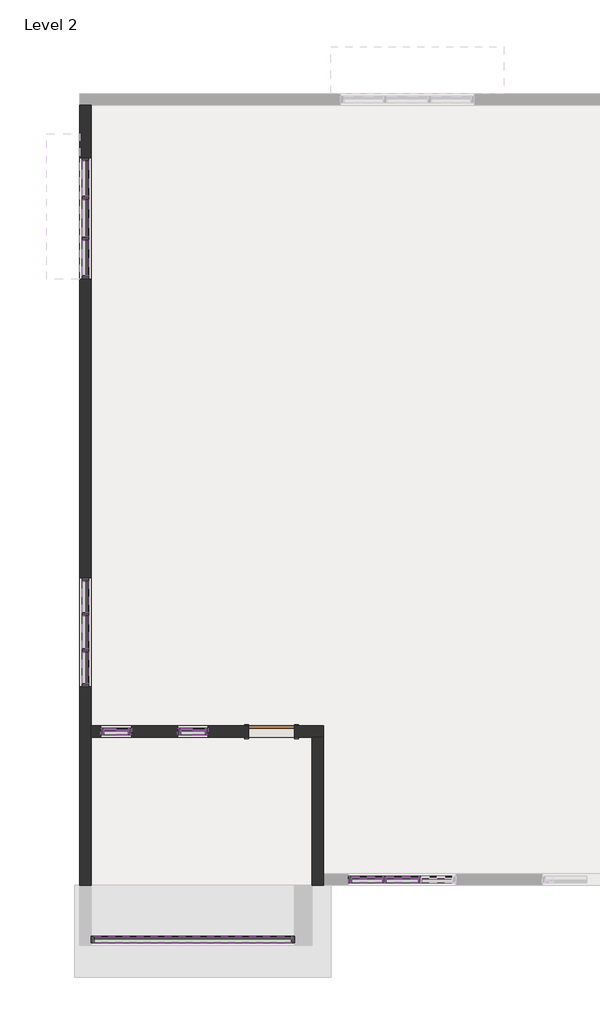
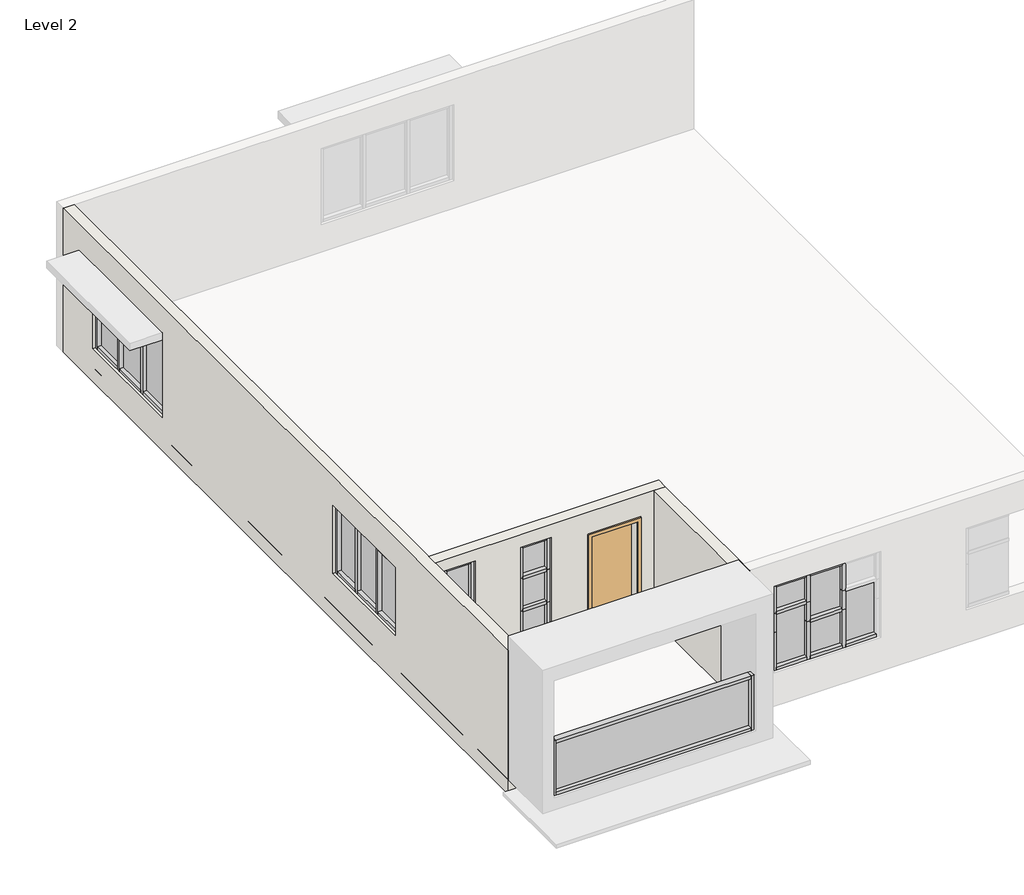
# One storey, part 1 of 2: 60 members, 18 plates, 3 walls, 1 door.
"""IFC4 building model written with IfcOpenShell, lengths in millimetres."""

from ifc_helpers import new_model, si_unit, frame, origin, place, context, project, spatial, polyline, outline, extrude, faceted_brep, transform, mapped, element, save
from components import door_a90ba1ad, member_3f0e0172, member_5215b92c, member_e53b78c9, member_f8dc38bf, member_504574e5, member_b70ee1cc, member_323df77c, member_86d06fe4, member_c0b2eca9, member_1f059faf, member_ce3cb600, member_25d88653, member_13f6f031, member_d2428cc8, member_166502d3, member_d74631f0, member_63be31b3, member_891d357d, member_df93ad89, member_28ac88d2, member_2030dc42, member_297e028d, member_b5a88f55, member_6ca94d07, member_46c3daae, system_panel_glazed_bdd26bb3, system_panel_glazed_84c2177b, system_panel_glazed_04707b35, system_panel_glazed_fe1d3f05, system_panel_glazed_483907af, system_panel_glazed_5a74f323, system_panel_glazed_03a03fc4, system_panel_glazed_c2563f89, system_panel_glazed_d3cf7d22, system_panel_glazed_f04aca20, system_panel_glazed_b3daaad5, system_panel_glazed_3e14b5a9, system_panel_glazed_68555a4f, system_panel_glazed_82e5a723

model = new_model("IFC4")

# Units and contexts
model_context = context("Model", 3, world=origin())
ifc_project = project(units=[si_unit("LENGTHUNIT", "METRE", prefix="MILLI")], contexts=[model_context])

# Site, building, storey
site = spatial("IfcSite", under=ifc_project)
building = spatial("IfcBuilding", under=site)
storey = spatial("IfcBuildingStorey", under=building, Name="Level 2", Elevation=3048.0)

# Door
placement = place(None, origin())
door_shape = door_a90ba1ad(model_context)
element("IfcDoor", 1, ObjectType="Single-Flush : 36\" x 84\"", at=placement, inside=storey, context=model_context, shape_type="MappedRepresentation", body=[
    mapped(door_shape, transform((-18035.6161422, -11856.2171312, 3429.0), x_axis=(-1.0, 0.0, 0.0), y_axis=(0.0, -1.0, 0.0), z_axis=(0.0, 0.0, 1.0))),
])

# Members
element("IfcMember", 2, ObjectType="Rectangular Mullion : 2.5\" x 5\" rectangular", at=placement, inside=storey, context=model_context, shape_type="SweptSolid", body=[
    extrude(outline(polyline([(-21553.5161422, -16047.2171312), (-21553.5161422, -15920.2171312), (-17641.9161422, -15920.2171312), (-17641.9161422, -16047.2171312), (-21553.5161422, -16047.2171312)])), frame((0.0, 0.0, 3616.9897637), z_axis=(0.0, 0.0, 1.0), x_axis=(1.0, 0.0, 0.0)), (0.0, 0.0, 1.0), 63.5),
])
member_shape = member_3f0e0172(model_context)
element("IfcMember", 3, ObjectType="Rectangular Mullion : 2.5\" x 5\" rectangular", at=placement, inside=storey, context=model_context, shape_type="MappedRepresentation", body=[
    mapped(member_shape, transform((-15057.4661422, -14789.9171312, 3757.8785057), x_axis=(0.0, 0.0, -1.0), y_axis=(0.0, -1.0, 0.0), z_axis=(-1.0, 0.0, 0.0))),
])
element("IfcMember", 4, ObjectType="Rectangular Mullion : 2.5\" x 5\" rectangular", at=placement, inside=storey, context=model_context, shape_type="MappedRepresentation", body=[
    mapped(member_shape, transform((-16448.1161422, -14789.9171312, 3757.8785057), x_axis=(0.0, 0.0, -1.0), y_axis=(0.0, -1.0, 0.0), z_axis=(-1.0, 0.0, 0.0))),
])
element("IfcMember", 5, ObjectType="Rectangular Mullion : 2.5\" x 5\" rectangular", at=placement, inside=storey, context=model_context, shape_type="MappedRepresentation", body=[
    mapped(member_shape, transform((-15832.1661422, -14789.9171312, 5583.6799972), x_axis=(0.0, 0.0, 1.0), y_axis=(0.0, -1.0, 0.0), z_axis=(1.0, 0.0, 0.0))),
])
member_2_shape = member_5215b92c(model_context)
element("IfcMember", 6, ObjectType="Rectangular Mullion : 2.5\" x 5\" rectangular", at=placement, inside=storey, context=model_context, shape_type="MappedRepresentation", body=[
    mapped(member_2_shape, transform((-15768.6661422, -14789.9171312, 3757.8785057), x_axis=(0.0, 0.0, -1.0), y_axis=(0.0, -1.0, 0.0), z_axis=(-1.0, 0.0, 0.0))),
])
element("IfcMember", 7, ObjectType="Rectangular Mullion : 2.5\" x 5\" rectangular", at=placement, inside=storey, context=model_context, shape_type="MappedRepresentation", body=[
    mapped(member_2_shape, transform((-15120.9661422, -14789.9171312, 5583.6799972), x_axis=(0.0, 0.0, 1.0), y_axis=(0.0, -1.0, 0.0), z_axis=(1.0, 0.0, 0.0))),
])
member_3_shape = member_e53b78c9(model_context)
element("IfcMember", 8, ObjectType="Rectangular Mullion : 2.5\" x 5\" rectangular", at=placement, inside=storey, context=model_context, shape_type="MappedRepresentation", body=[
    mapped(member_3_shape, transform((-15120.9661422, -14789.9171312, 4569.3458353), x_axis=(0.0, 0.0, 1.0), y_axis=(0.0, -1.0, 0.0), z_axis=(1.0, 0.0, 0.0))),
])
member_4_shape = member_f8dc38bf(model_context)
element("IfcMember", 9, ObjectType="Rectangular Mullion : 2.5\" x 5\" rectangular", at=placement, inside=storey, context=model_context, shape_type="MappedRepresentation", body=[
    mapped(member_4_shape, transform((-15832.1661422, -14789.9171312, 4975.0795001), x_axis=(0.0, 0.0, 1.0), y_axis=(0.0, -1.0, 0.0), z_axis=(1.0, 0.0, 0.0))),
])
member_5_shape = member_504574e5(model_context)
element("IfcMember", 10, ObjectType="Rectangular Mullion : 2.5\" x 5\" rectangular", at=placement, inside=storey, context=model_context, shape_type="MappedRepresentation", body=[
    mapped(member_5_shape, transform((-21426.5161422, -11856.2171312, 4991.9456117), x_axis=(-1.0, 0.0, 0.0), y_axis=(0.0, -1.0, 0.0), z_axis=(0.0, 0.0, 1.0))),
])
member_6_shape = member_b70ee1cc(model_context)
element("IfcMember", 11, ObjectType="Rectangular Mullion : 2.5\" x 5\" rectangular", at=placement, inside=storey, context=model_context, shape_type="MappedRepresentation", body=[
    mapped(member_6_shape, transform((-21426.5161422, -11856.2171312, 5855.5456117), x_axis=(-1.0, 0.0, 0.0), y_axis=(0.0, -1.0, 0.0), z_axis=(0.0, 0.0, 1.0))),
])
member_7_shape = member_323df77c(model_context)
element("IfcMember", 12, ObjectType="Rectangular Mullion : 2.5\" x 5\" rectangular", at=placement, inside=storey, context=model_context, shape_type="MappedRepresentation", body=[
    mapped(member_7_shape, transform((-20880.4161422, -11856.2171312, 4991.9456117), x_axis=(0.0, 0.0, 1.0), y_axis=(0.0, -1.0, 0.0), z_axis=(1.0, 0.0, 0.0))),
])
element("IfcMember", 13, ObjectType="Rectangular Mullion : 2.5\" x 5\" rectangular", at=placement, inside=storey, context=model_context, shape_type="MappedRepresentation", body=[
    mapped(member_7_shape, transform((-20880.4161422, -11856.2171312, 4416.0583974), x_axis=(0.0, 0.0, 1.0), y_axis=(0.0, -1.0, 0.0), z_axis=(1.0, 0.0, 0.0))),
])
element("IfcMember", 14, ObjectType="Rectangular Mullion : 2.5\" x 5\" rectangular", at=placement, inside=storey, context=model_context, shape_type="MappedRepresentation", body=[
    mapped(member_7_shape, transform((-19356.4161422, -11856.2171312, 5127.093488), x_axis=(0.0, 0.0, 1.0), y_axis=(0.0, -1.0, 0.0), z_axis=(1.0, 0.0, 0.0))),
])
element("IfcMember", 15, ObjectType="Rectangular Mullion : 2.5\" x 5\" rectangular", at=placement, inside=storey, context=model_context, shape_type="MappedRepresentation", body=[
    mapped(member_7_shape, transform((-19356.4161422, -11856.2171312, 4429.6158671), x_axis=(0.0, 0.0, 1.0), y_axis=(0.0, -1.0, 0.0), z_axis=(1.0, 0.0, 0.0))),
])
member_8_shape = member_86d06fe4(model_context)
element("IfcMember", 16, ObjectType="Rectangular Mullion : 2.5\" x 5\" rectangular", at=placement, inside=storey, context=model_context, shape_type="MappedRepresentation", body=[
    mapped(member_8_shape, transform((-20880.4161422, -11856.2171312, 5855.5456117), x_axis=(0.0, 0.0, 1.0), y_axis=(0.0, -1.0, 0.0), z_axis=(1.0, 0.0, 0.0))),
])
element("IfcMember", 17, ObjectType="Rectangular Mullion : 2.5\" x 5\" rectangular", at=placement, inside=storey, context=model_context, shape_type="MappedRepresentation", body=[
    mapped(member_8_shape, transform((-19356.4161422, -11856.2171312, 5824.5711089), x_axis=(0.0, 0.0, 1.0), y_axis=(0.0, -1.0, 0.0), z_axis=(1.0, 0.0, 0.0))),
])
element("IfcMember", 18, ObjectType="Rectangular Mullion : 2.5\" x 5\" rectangular", at=placement, inside=storey, context=model_context, shape_type="MappedRepresentation", body=[
    mapped(member_5_shape, transform((-20816.9161422, -11856.2171312, 4416.0583974), x_axis=(1.0, 0.0, 0.0), y_axis=(0.0, -1.0, 0.0), z_axis=(0.0, 0.0, -1.0))),
])
element("IfcMember", 19, ObjectType="Rectangular Mullion : 2.5\" x 5\" rectangular", at=placement, inside=storey, context=model_context, shape_type="MappedRepresentation", body=[
    mapped(member_6_shape, transform((-20816.9161422, -11856.2171312, 4991.9456117), x_axis=(1.0, 0.0, 0.0), y_axis=(0.0, -1.0, 0.0), z_axis=(0.0, 0.0, -1.0))),
])
element("IfcMember", 20, ObjectType="Rectangular Mullion : 2.5\" x 5\" rectangular", at=placement, inside=storey, context=model_context, shape_type="MappedRepresentation", body=[
    mapped(member_8_shape, transform((-21363.0161422, -11856.2171312, 3840.1711831), x_axis=(0.0, 0.0, -1.0), y_axis=(0.0, -1.0, 0.0), z_axis=(-1.0, 0.0, 0.0))),
])
element("IfcMember", 21, ObjectType="Rectangular Mullion : 2.5\" x 5\" rectangular", at=placement, inside=storey, context=model_context, shape_type="MappedRepresentation", body=[
    mapped(member_8_shape, transform((-19839.0161422, -11856.2171312, 3732.1382463), x_axis=(0.0, 0.0, -1.0), y_axis=(0.0, -1.0, 0.0), z_axis=(-1.0, 0.0, 0.0))),
])
element("IfcMember", 22, ObjectType="Rectangular Mullion : 2.5\" x 5\" rectangular", at=placement, inside=storey, context=model_context, shape_type="MappedRepresentation", body=[
    mapped(member_5_shape, transform((-21426.5161422, -11856.2171312, 4416.0583974), x_axis=(-1.0, 0.0, 0.0), y_axis=(0.0, -1.0, 0.0), z_axis=(0.0, 0.0, 1.0))),
])
element("IfcMember", 23, ObjectType="Rectangular Mullion : 2.5\" x 5\" rectangular", at=placement, inside=storey, context=model_context, shape_type="MappedRepresentation", body=[
    mapped(member_5_shape, transform((-20816.9161422, -11856.2171312, 3840.1711831), x_axis=(1.0, 0.0, 0.0), y_axis=(0.0, -1.0, 0.0), z_axis=(0.0, 0.0, -1.0))),
])
member_9_shape = member_c0b2eca9(model_context)
element("IfcMember", 24, ObjectType="Rectangular Mullion : 2.5\" x 5\" rectangular", at=placement, inside=storey, context=model_context, shape_type="MappedRepresentation", body=[
    mapped(member_9_shape, transform((-19902.5161422, -11856.2171312, 5824.5711089), x_axis=(-1.0, 0.0, 0.0), y_axis=(0.0, -1.0, 0.0), z_axis=(0.0, 0.0, 1.0))),
])
element("IfcMember", 25, ObjectType="Rectangular Mullion : 2.5\" x 5\" rectangular", at=placement, inside=storey, context=model_context, shape_type="MappedRepresentation", body=[
    mapped(member_9_shape, transform((-19902.5161422, -11856.2171312, 5127.093488), x_axis=(-1.0, 0.0, 0.0), y_axis=(0.0, -1.0, 0.0), z_axis=(0.0, 0.0, 1.0))),
])
element("IfcMember", 26, ObjectType="Rectangular Mullion : 2.5\" x 5\" rectangular", at=placement, inside=storey, context=model_context, shape_type="MappedRepresentation", body=[
    mapped(member_9_shape, transform((-19902.5161422, -11856.2171312, 4429.6158671), x_axis=(-1.0, 0.0, 0.0), y_axis=(0.0, -1.0, 0.0), z_axis=(0.0, 0.0, 1.0))),
])
element("IfcMember", 27, ObjectType="Rectangular Mullion : 2.5\" x 5\" rectangular", at=placement, inside=storey, context=model_context, shape_type="MappedRepresentation", body=[
    mapped(member_9_shape, transform((-19292.9161422, -11856.2171312, 4429.6158671), x_axis=(1.0, 0.0, 0.0), y_axis=(0.0, -1.0, 0.0), z_axis=(0.0, 0.0, -1.0))),
])
element("IfcMember", 28, ObjectType="Rectangular Mullion : 2.5\" x 5\" rectangular", at=placement, inside=storey, context=model_context, shape_type="MappedRepresentation", body=[
    mapped(member_9_shape, transform((-19292.9161422, -11856.2171312, 5127.093488), x_axis=(1.0, 0.0, 0.0), y_axis=(0.0, -1.0, 0.0), z_axis=(0.0, 0.0, -1.0))),
])
element("IfcMember", 29, ObjectType="Rectangular Mullion : 2.5\" x 5\" rectangular", at=placement, inside=storey, context=model_context, shape_type="MappedRepresentation", body=[
    mapped(member_9_shape, transform((-19292.9161422, -11856.2171312, 3732.1382463), x_axis=(1.0, 0.0, 0.0), y_axis=(0.0, -1.0, 0.0), z_axis=(0.0, 0.0, -1.0))),
])
member_10_shape = member_1f059faf(model_context)
element("IfcMember", 30, ObjectType="Rectangular Mullion : 2.5\" x 5\" rectangular", at=placement, inside=storey, context=model_context, shape_type="MappedRepresentation", body=[
    mapped(member_10_shape, transform((-16511.6161422, -14789.9171312, 4569.3458353), x_axis=(-1.0, 0.0, 0.0), y_axis=(0.0, -1.0, 0.0), z_axis=(0.0, 0.0, 1.0))),
])
member_11_shape = member_ce3cb600(model_context)
element("IfcMember", 31, ObjectType="Rectangular Mullion : 2.5\" x 5\" rectangular", at=placement, inside=storey, context=model_context, shape_type="MappedRepresentation", body=[
    mapped(member_11_shape, transform((-15800.4161422, -14789.9171312, 4975.0795001), x_axis=(1.0, 0.0, 0.0), y_axis=(0.0, -1.0, 0.0), z_axis=(0.0, 0.0, -1.0))),
])
element("IfcMember", 32, ObjectType="Rectangular Mullion : 2.5\" x 5\" rectangular", at=placement, inside=storey, context=model_context, shape_type="MappedRepresentation", body=[
    mapped(member_11_shape, transform((-15089.2161422, -14789.9171312, 4975.0795001), x_axis=(1.0, 0.0, 0.0), y_axis=(0.0, -1.0, 0.0), z_axis=(0.0, 0.0, -1.0))),
])
member_12_shape = member_25d88653(model_context)
element("IfcMember", 33, ObjectType="Rectangular Mullion : 2.5\" x 5\" rectangular", at=placement, inside=storey, context=model_context, shape_type="MappedRepresentation", body=[
    mapped(member_12_shape, transform((-16511.6161422, -14789.9171312, 4975.0795001), x_axis=(-1.0, 0.0, 0.0), y_axis=(0.0, -1.0, 0.0), z_axis=(0.0, 0.0, 1.0))),
])
member_13_shape = member_13f6f031(model_context)
element("IfcMember", 34, ObjectType="Rectangular Mullion : 2.5\" x 5\" rectangular", at=placement, inside=storey, context=model_context, shape_type="MappedRepresentation", body=[
    mapped(member_13_shape, transform((-16511.6161422, -14789.9171312, 5583.6799972), x_axis=(-1.0, 0.0, 0.0), y_axis=(0.0, -1.0, 0.0), z_axis=(0.0, 0.0, 1.0))),
])
member_14_shape = member_d2428cc8(model_context)
element("IfcMember", 35, ObjectType="Rectangular Mullion : 2.5\" x 5\" rectangular", at=placement, inside=storey, context=model_context, shape_type="MappedRepresentation", body=[
    mapped(member_14_shape, transform((-15800.4161422, -14789.9171312, 4569.3458353), x_axis=(1.0, 0.0, 0.0), y_axis=(0.0, -1.0, 0.0), z_axis=(0.0, 0.0, -1.0))),
])
element("IfcMember", 36, ObjectType="Rectangular Mullion : 2.5\" x 5\" rectangular", at=placement, inside=storey, context=model_context, shape_type="MappedRepresentation", body=[
    mapped(member_14_shape, transform((-15089.2161422, -14789.9171312, 4569.3458353), x_axis=(1.0, 0.0, 0.0), y_axis=(0.0, -1.0, 0.0), z_axis=(0.0, 0.0, -1.0))),
])
member_15_shape = member_166502d3(model_context)
element("IfcMember", 37, ObjectType="Rectangular Mullion : 2.5\" x 5\" rectangular", at=placement, inside=storey, context=model_context, shape_type="MappedRepresentation", body=[
    mapped(member_15_shape, transform((-15800.4161422, -14789.9171312, 3757.8785057), x_axis=(1.0, 0.0, 0.0), y_axis=(0.0, -1.0, 0.0), z_axis=(0.0, 0.0, -1.0))),
])
element("IfcMember", 38, ObjectType="Rectangular Mullion : 2.5\" x 5\" rectangular", at=placement, inside=storey, context=model_context, shape_type="MappedRepresentation", body=[
    mapped(member_15_shape, transform((-15089.2161422, -14789.9171312, 3757.8785057), x_axis=(1.0, 0.0, 0.0), y_axis=(0.0, -1.0, 0.0), z_axis=(0.0, 0.0, -1.0))),
])
member_16_shape = member_d74631f0(model_context)
element("IfcMember", 39, ObjectType="Rectangular Mullion : 2.5\" x 5\" rectangular", at=placement, inside=storey, context=model_context, shape_type="MappedRepresentation", body=[
    mapped(member_16_shape, transform((-21617.0161422, -15983.7171312, 4779.1840663), x_axis=(-1.0, 0.0, 0.0), y_axis=(0.0, -1.0, 0.0), z_axis=(0.0, 0.0, 1.0))),
])
member_17_shape = member_63be31b3(model_context)
element("IfcMember", 40, ObjectType="Rectangular Mullion : 2.5\" x 5\" rectangular", at=placement, inside=storey, context=model_context, shape_type="MappedRepresentation", body=[
    mapped(member_17_shape, transform((-17641.9161422, -15983.7171312, 4779.1840663), x_axis=(0.0, 0.0, 1.0), y_axis=(0.0, -1.0, 0.0), z_axis=(1.0, 0.0, 0.0))),
])
element("IfcMember", 41, ObjectType="Rectangular Mullion : 2.5\" x 5\" rectangular", at=placement, inside=storey, context=model_context, shape_type="MappedRepresentation", body=[
    mapped(member_16_shape, transform((-17578.4161422, -15983.7171312, 3616.9897637), x_axis=(1.0, 0.0, 0.0), y_axis=(0.0, -1.0, 0.0), z_axis=(0.0, 0.0, -1.0))),
])
member_18_shape = member_891d357d(model_context)
element("IfcMember", 42, ObjectType="Rectangular Mullion : 2.5\" x 5\" rectangular", at=placement, inside=storey, context=model_context, shape_type="MappedRepresentation", body=[
    mapped(member_18_shape, transform((-21731.3161422, -2046.5619465, 5394.6234092), x_axis=(0.0, 0.0, 1.0), y_axis=(-1.0, 0.0, 0.0), z_axis=(0.0, -1.0, 0.0))),
])
member_19_shape = member_df93ad89(model_context)
element("IfcMember", 43, ObjectType="Rectangular Mullion : 2.5\" x 5\" rectangular", at=placement, inside=storey, context=model_context, shape_type="MappedRepresentation", body=[
    mapped(member_19_shape, transform((-21731.3161422, -1242.850651, 5394.6234092), x_axis=(0.0, 0.0, 1.0), y_axis=(-1.0, 0.0, 0.0), z_axis=(0.0, -1.0, 0.0))),
])
element("IfcMember", 44, ObjectType="Rectangular Mullion : 2.5\" x 5\" rectangular", at=placement, inside=storey, context=model_context, shape_type="MappedRepresentation", body=[
    mapped(member_19_shape, transform((-21731.3161422, -2818.523242, 5394.6234092), x_axis=(0.0, 0.0, 1.0), y_axis=(-1.0, 0.0, 0.0), z_axis=(0.0, -1.0, 0.0))),
])
member_20_shape = member_28ac88d2(model_context)
element("IfcMember", 45, ObjectType="Rectangular Mullion : 2.5\" x 5\" rectangular", at=placement, inside=storey, context=model_context, shape_type="MappedRepresentation", body=[
    mapped(member_20_shape, transform((-21731.3161422, -1274.600651, 3744.6696431), x_axis=(0.0, -1.0, 0.0), y_axis=(-1.0, 0.0, 0.0), z_axis=(0.0, 0.0, -1.0))),
])
element("IfcMember", 46, ObjectType="Rectangular Mullion : 2.5\" x 5\" rectangular", at=placement, inside=storey, context=model_context, shape_type="MappedRepresentation", body=[
    mapped(member_20_shape, transform((-21731.3161422, -2078.3119465, 3744.6696431), x_axis=(0.0, -1.0, 0.0), y_axis=(-1.0, 0.0, 0.0), z_axis=(0.0, 0.0, -1.0))),
])
element("IfcMember", 47, ObjectType="Rectangular Mullion : 2.5\" x 5\" rectangular", at=placement, inside=storey, context=model_context, shape_type="MappedRepresentation", body=[
    mapped(member_19_shape, transform((-21731.3161422, -2110.0619465, 3744.6696431), x_axis=(0.0, 0.0, -1.0), y_axis=(-1.0, 0.0, 0.0), z_axis=(0.0, 1.0, 0.0))),
])
element("IfcMember", 48, ObjectType="Rectangular Mullion : 2.5\" x 5\" rectangular", at=placement, inside=storey, context=model_context, shape_type="MappedRepresentation", body=[
    mapped(member_19_shape, transform((-21731.3161422, -534.3893556, 3744.6696431), x_axis=(0.0, 0.0, -1.0), y_axis=(-1.0, 0.0, 0.0), z_axis=(0.0, 1.0, 0.0))),
])
element("IfcMember", 49, ObjectType="Rectangular Mullion : 2.5\" x 5\" rectangular", at=placement, inside=storey, context=model_context, shape_type="MappedRepresentation", body=[
    mapped(member_18_shape, transform((-21731.3161422, -1306.350651, 3744.6696431), x_axis=(0.0, 0.0, -1.0), y_axis=(-1.0, 0.0, 0.0), z_axis=(0.0, 1.0, 0.0))),
])
member_21_shape = member_2030dc42(model_context)
element("IfcMember", 50, ObjectType="Rectangular Mullion : 2.5\" x 5\" rectangular", at=placement, inside=storey, context=model_context, shape_type="MappedRepresentation", body=[
    mapped(member_21_shape, transform((-21731.3161422, -2882.023242, 3744.6696431), x_axis=(0.0, -1.0, 0.0), y_axis=(-1.0, 0.0, 0.0), z_axis=(0.0, 0.0, -1.0))),
])
element("IfcMember", 51, ObjectType="Rectangular Mullion : 2.5\" x 5\" rectangular", at=placement, inside=storey, context=model_context, shape_type="MappedRepresentation", body=[
    mapped(member_21_shape, transform((-21731.3161422, -470.8893556, 5394.6234092), x_axis=(0.0, 1.0, 0.0), y_axis=(-1.0, 0.0, 0.0), z_axis=(0.0, 0.0, 1.0))),
])
member_22_shape = member_297e028d(model_context)
element("IfcMember", 52, ObjectType="Rectangular Mullion : 2.5\" x 5\" rectangular", at=placement, inside=storey, context=model_context, shape_type="MappedRepresentation", body=[
    mapped(member_22_shape, transform((-21731.3161422, -10215.8004645, 5474.4213477), x_axis=(0.0, 0.0, 1.0), y_axis=(-1.0, 0.0, 0.0), z_axis=(0.0, -1.0, 0.0))),
])
member_23_shape = member_b5a88f55(model_context)
element("IfcMember", 53, ObjectType="Rectangular Mullion : 2.5\" x 5\" rectangular", at=placement, inside=storey, context=model_context, shape_type="MappedRepresentation", body=[
    mapped(member_23_shape, transform((-21731.3161422, -9496.1337979, 5474.4213477), x_axis=(0.0, 0.0, 1.0), y_axis=(-1.0, 0.0, 0.0), z_axis=(0.0, -1.0, 0.0))),
])
element("IfcMember", 54, ObjectType="Rectangular Mullion : 2.5\" x 5\" rectangular", at=placement, inside=storey, context=model_context, shape_type="MappedRepresentation", body=[
    mapped(member_23_shape, transform((-21731.3161422, -10903.7171312, 5474.4213477), x_axis=(0.0, 0.0, 1.0), y_axis=(-1.0, 0.0, 0.0), z_axis=(0.0, -1.0, 0.0))),
])
member_24_shape = member_6ca94d07(model_context)
element("IfcMember", 55, ObjectType="Rectangular Mullion : 2.5\" x 5\" rectangular", at=placement, inside=storey, context=model_context, shape_type="MappedRepresentation", body=[
    mapped(member_24_shape, transform((-21731.3161422, -9527.8837979, 4032.1019574), x_axis=(0.0, -1.0, 0.0), y_axis=(-1.0, 0.0, 0.0), z_axis=(0.0, 0.0, -1.0))),
])
element("IfcMember", 56, ObjectType="Rectangular Mullion : 2.5\" x 5\" rectangular", at=placement, inside=storey, context=model_context, shape_type="MappedRepresentation", body=[
    mapped(member_24_shape, transform((-21731.3161422, -10247.5504645, 4032.1019574), x_axis=(0.0, -1.0, 0.0), y_axis=(-1.0, 0.0, 0.0), z_axis=(0.0, 0.0, -1.0))),
])
element("IfcMember", 57, ObjectType="Rectangular Mullion : 2.5\" x 5\" rectangular", at=placement, inside=storey, context=model_context, shape_type="MappedRepresentation", body=[
    mapped(member_23_shape, transform((-21731.3161422, -10279.3004645, 4032.1019574), x_axis=(0.0, 0.0, -1.0), y_axis=(-1.0, 0.0, 0.0), z_axis=(0.0, 1.0, 0.0))),
])
element("IfcMember", 58, ObjectType="Rectangular Mullion : 2.5\" x 5\" rectangular", at=placement, inside=storey, context=model_context, shape_type="MappedRepresentation", body=[
    mapped(member_23_shape, transform((-21731.3161422, -8871.7171312, 4032.1019574), x_axis=(0.0, 0.0, -1.0), y_axis=(-1.0, 0.0, 0.0), z_axis=(0.0, 1.0, 0.0))),
])
element("IfcMember", 59, ObjectType="Rectangular Mullion : 2.5\" x 5\" rectangular", at=placement, inside=storey, context=model_context, shape_type="MappedRepresentation", body=[
    mapped(member_22_shape, transform((-21731.3161422, -9559.6337979, 4032.1019574), x_axis=(0.0, 0.0, -1.0), y_axis=(-1.0, 0.0, 0.0), z_axis=(0.0, 1.0, 0.0))),
])
member_25_shape = member_46c3daae(model_context)
element("IfcMember", 60, ObjectType="Rectangular Mullion : 2.5\" x 5\" rectangular", at=placement, inside=storey, context=model_context, shape_type="MappedRepresentation", body=[
    mapped(member_25_shape, transform((-21731.3161422, -10967.2171312, 4032.1019574), x_axis=(0.0, -1.0, 0.0), y_axis=(-1.0, 0.0, 0.0), z_axis=(0.0, 0.0, -1.0))),
])
element("IfcMember", 61, ObjectType="Rectangular Mullion : 2.5\" x 5\" rectangular", at=placement, inside=storey, context=model_context, shape_type="MappedRepresentation", body=[
    mapped(member_25_shape, transform((-21731.3161422, -8808.2171312, 5474.4213477), x_axis=(0.0, 1.0, 0.0), y_axis=(-1.0, 0.0, 0.0), z_axis=(0.0, 0.0, 1.0))),
])

# Plates
system_panel_glazed_shape = system_panel_glazed_bdd26bb3(model_context)
element("IfcPlate", 62, ObjectType="System Panel : Glazed", at=placement, inside=storey, context=model_context, shape_type="MappedRepresentation", body=[
    mapped(system_panel_glazed_shape, transform((-21121.7161422, -11856.2171312, 5023.6956117), x_axis=(1.0, 0.0, 0.0), y_axis=(0.0, 1.0, 0.0), z_axis=(0.0, 0.0, 1.0))),
])
system_panel_glazed_2_shape = system_panel_glazed_84c2177b(model_context)
element("IfcPlate", 63, ObjectType="System Panel : Glazed", at=placement, inside=storey, context=model_context, shape_type="MappedRepresentation", body=[
    mapped(system_panel_glazed_2_shape, transform((-21121.7161422, -11856.2171312, 4447.8083974), x_axis=(1.0, 0.0, 0.0), y_axis=(0.0, 1.0, 0.0), z_axis=(0.0, 0.0, 1.0))),
])
system_panel_glazed_3_shape = system_panel_glazed_04707b35(model_context)
element("IfcPlate", 64, ObjectType="System Panel : Glazed", at=placement, inside=storey, context=model_context, shape_type="MappedRepresentation", body=[
    mapped(system_panel_glazed_3_shape, transform((-21121.7161422, -11856.2171312, 3903.6711831), x_axis=(1.0, 0.0, 0.0), y_axis=(0.0, 1.0, 0.0), z_axis=(0.0, 0.0, 1.0))),
])
system_panel_glazed_4_shape = system_panel_glazed_fe1d3f05(model_context)
element("IfcPlate", 65, ObjectType="System Panel : Glazed", at=placement, inside=storey, context=model_context, shape_type="MappedRepresentation", body=[
    mapped(system_panel_glazed_4_shape, transform((-19597.7161422, -11856.2171312, 3795.6382463), x_axis=(1.0, 0.0, 0.0), y_axis=(0.0, 1.0, 0.0), z_axis=(0.0, 0.0, 1.0))),
])
element("IfcPlate", 66, ObjectType="System Panel : Glazed", at=placement, inside=storey, context=model_context, shape_type="MappedRepresentation", body=[
    mapped(system_panel_glazed_4_shape, transform((-19597.7161422, -11856.2171312, 5158.843488), x_axis=(1.0, 0.0, 0.0), y_axis=(0.0, 1.0, 0.0), z_axis=(0.0, 0.0, 1.0))),
])
system_panel_glazed_5_shape = system_panel_glazed_483907af(model_context)
element("IfcPlate", 67, ObjectType="System Panel : Glazed", at=placement, inside=storey, context=model_context, shape_type="MappedRepresentation", body=[
    mapped(system_panel_glazed_5_shape, transform((-19597.7161422, -11856.2171312, 4461.3658671), x_axis=(1.0, 0.0, 0.0), y_axis=(0.0, 1.0, 0.0), z_axis=(0.0, 0.0, 1.0))),
])
system_panel_glazed_6_shape = system_panel_glazed_5a74f323(model_context)
element("IfcPlate", 68, ObjectType="System Panel : Glazed", at=placement, inside=storey, context=model_context, shape_type="MappedRepresentation", body=[
    mapped(system_panel_glazed_6_shape, transform((-16140.1411422, -14789.9171312, 3821.3785057), x_axis=(1.0, 0.0, 0.0), y_axis=(0.0, 1.0, 0.0), z_axis=(0.0, 0.0, 1.0))),
])
element("IfcPlate", 69, ObjectType="System Panel : Glazed", at=placement, inside=storey, context=model_context, shape_type="MappedRepresentation", body=[
    mapped(system_panel_glazed_6_shape, transform((-14749.4911422, -14789.9171312, 3821.3785057), x_axis=(1.0, 0.0, 0.0), y_axis=(0.0, 1.0, 0.0), z_axis=(0.0, 0.0, 1.0))),
])
system_panel_glazed_7_shape = system_panel_glazed_03a03fc4(model_context)
element("IfcPlate", 70, ObjectType="System Panel : Glazed", at=placement, inside=storey, context=model_context, shape_type="MappedRepresentation", body=[
    mapped(system_panel_glazed_7_shape, transform((-16140.1411422, -14789.9171312, 5006.8295001), x_axis=(1.0, 0.0, 0.0), y_axis=(0.0, 1.0, 0.0), z_axis=(0.0, 0.0, 1.0))),
])
system_panel_glazed_8_shape = system_panel_glazed_c2563f89(model_context)
element("IfcPlate", 71, ObjectType="System Panel : Glazed", at=placement, inside=storey, context=model_context, shape_type="MappedRepresentation", body=[
    mapped(system_panel_glazed_8_shape, transform((-15444.8161422, -14789.9171312, 3821.3785057), x_axis=(1.0, 0.0, 0.0), y_axis=(0.0, 1.0, 0.0), z_axis=(0.0, 0.0, 1.0))),
])
system_panel_glazed_9_shape = system_panel_glazed_d3cf7d22(model_context)
element("IfcPlate", 72, ObjectType="System Panel : Glazed", at=placement, inside=storey, context=model_context, shape_type="MappedRepresentation", body=[
    mapped(system_panel_glazed_9_shape, transform((-15444.8161422, -14789.9171312, 4601.0958353), x_axis=(1.0, 0.0, 0.0), y_axis=(0.0, 1.0, 0.0), z_axis=(0.0, 0.0, 1.0))),
])
system_panel_glazed_10_shape = system_panel_glazed_f04aca20(model_context)
element("IfcPlate", 73, ObjectType="System Panel : Glazed", at=placement, inside=storey, context=model_context, shape_type="MappedRepresentation", body=[
    mapped(system_panel_glazed_10_shape, transform((-19597.7161422, -15983.7171312, 3680.4897637), x_axis=(1.0, 0.0, 0.0), y_axis=(0.0, 1.0, 0.0), z_axis=(0.0, 0.0, 1.0))),
])
system_panel_glazed_11_shape = system_panel_glazed_b3daaad5(model_context)
element("IfcPlate", 74, ObjectType="System Panel : Glazed", at=placement, inside=storey, context=model_context, shape_type="MappedRepresentation", body=[
    mapped(system_panel_glazed_11_shape, transform((-21731.3161422, -888.6200033, 3808.1696431), x_axis=(0.0, -1.0, 0.0), y_axis=(1.0, 0.0, 0.0), z_axis=(0.0, 0.0, 1.0))),
])
element("IfcPlate", 75, ObjectType="System Panel : Glazed", at=placement, inside=storey, context=model_context, shape_type="MappedRepresentation", body=[
    mapped(system_panel_glazed_11_shape, transform((-21731.3161422, -2464.2925943, 3808.1696431), x_axis=(0.0, -1.0, 0.0), y_axis=(1.0, 0.0, 0.0), z_axis=(0.0, 0.0, 1.0))),
])
system_panel_glazed_12_shape = system_panel_glazed_3e14b5a9(model_context)
element("IfcPlate", 76, ObjectType="System Panel : Glazed", at=placement, inside=storey, context=model_context, shape_type="MappedRepresentation", body=[
    mapped(system_panel_glazed_12_shape, transform((-21731.3161422, -1676.4562988, 3808.1696431), x_axis=(0.0, -1.0, 0.0), y_axis=(1.0, 0.0, 0.0), z_axis=(0.0, 0.0, 1.0))),
])
system_panel_glazed_13_shape = system_panel_glazed_68555a4f(model_context)
element("IfcPlate", 77, ObjectType="System Panel : Glazed", at=placement, inside=storey, context=model_context, shape_type="MappedRepresentation", body=[
    mapped(system_panel_glazed_13_shape, transform((-21731.3161422, -9183.9254645, 4095.6019574), x_axis=(0.0, -1.0, 0.0), y_axis=(1.0, 0.0, 0.0), z_axis=(0.0, 0.0, 1.0))),
])
element("IfcPlate", 78, ObjectType="System Panel : Glazed", at=placement, inside=storey, context=model_context, shape_type="MappedRepresentation", body=[
    mapped(system_panel_glazed_13_shape, transform((-21731.3161422, -10591.5087979, 4095.6019574), x_axis=(0.0, -1.0, 0.0), y_axis=(1.0, 0.0, 0.0), z_axis=(0.0, 0.0, 1.0))),
])
system_panel_glazed_14_shape = system_panel_glazed_82e5a723(model_context)
element("IfcPlate", 79, ObjectType="System Panel : Glazed", at=placement, inside=storey, context=model_context, shape_type="MappedRepresentation", body=[
    mapped(system_panel_glazed_14_shape, transform((-21731.3161422, -9887.7171312, 4095.6019574), x_axis=(0.0, -1.0, 0.0), y_axis=(1.0, 0.0, 0.0), z_axis=(0.0, 0.0, 1.0))),
])

# Walls
element("IfcWall", 80, ObjectType="9\"", at=placement, inside=storey, context=model_context, shape_type="Brep", body=[
    faceted_brep([(-21617.0161422, -14904.2171312, 3048.0), (-21617.0161422, -11970.5171312, 3048.0), (-21617.0161422, -11741.9171312, 3048.0), (-21617.0161422, 564.3828688, 3048.0), (-21617.0161422, 564.3828688, 6096.0), (-21617.0161422, -11741.9171312, 6096.0), (-21617.0161422, -11970.5171312, 6096.0), (-21617.0161422, -14904.2171312, 6096.0), (-21617.0161422, -470.8893556, 5394.6234092), (-21617.0161422, -470.8893556, 3744.6696431), (-21617.0161422, -2882.023242, 3744.6696431), (-21617.0161422, -2882.023242, 5394.6234092), (-21617.0161422, -8808.2171312, 5474.4213477), (-21617.0161422, -8808.2171312, 4032.1019574), (-21617.0161422, -10967.2171312, 4032.1019574), (-21617.0161422, -10967.2171312, 5474.4213477), (-21845.6161422, 564.3828688, 3048.0), (-21845.6161422, -14904.2171312, 3048.0), (-21845.6161422, -14904.2171312, 6096.0), (-21845.6161422, 564.3828688, 6096.0), (-21845.6161422, -470.8893556, 3744.6696431), (-21845.6161422, -470.8893556, 5394.6234092), (-21845.6161422, -2882.023242, 5394.6234092), (-21845.6161422, -2882.023242, 3744.6696431), (-21845.6161422, -8808.2171312, 4032.1019574), (-21845.6161422, -8808.2171312, 5474.4213477), (-21845.6161422, -10967.2171312, 5474.4213477), (-21845.6161422, -10967.2171312, 4032.1019574)], [[[0, 1, 2, 3, 4, 5, 6, 7], [8, 9, 10, 11], [12, 13, 14, 15]], [[16, 17, 18, 19], [20, 21, 22, 23], [24, 25, 26, 27]], [[3, 2, 1, 0, 17, 16]], [[7, 6, 5, 4, 19, 18]], [[0, 7, 18, 17]], [[4, 3, 16, 19]], [[20, 9, 8, 21]], [[21, 8, 11, 22]], [[22, 11, 10, 23]], [[9, 20, 23, 10]], [[12, 25, 24, 13]], [[25, 12, 15, 26]], [[26, 15, 14, 27]], [[13, 24, 27, 14]]]),
])
element("IfcWall", 81, ObjectType="9\"", at=placement, inside=storey, context=model_context, shape_type="Brep", body=[
    faceted_brep([(-21617.0161422, -11970.5171312, 3048.0), (-17235.5161422, -11970.5171312, 3048.0), (-17006.9161422, -11970.5171312, 3048.0), (-17006.9161422, -11970.5171312, 6096.0), (-17235.5161422, -11970.5171312, 6096.0), (-21617.0161422, -11970.5171312, 6096.0), (-17578.4161422, -11970.5171312, 3429.0), (-18492.8161422, -11970.5171312, 3429.0), (-18492.8161422, -11970.5171312, 5562.6), (-17578.4161422, -11970.5171312, 5562.6), (-21426.5161422, -11970.5171312, 3840.1711831), (-21426.5161422, -11970.5171312, 5855.5456117), (-20816.9161422, -11970.5171312, 5855.5456117), (-20816.9161422, -11970.5171312, 3840.1711831), (-19902.5161422, -11970.5171312, 3732.1382463), (-19902.5161422, -11970.5171312, 5824.5711089), (-19292.9161422, -11970.5171312, 5824.5711089), (-19292.9161422, -11970.5171312, 3732.1382463), (-17006.9161422, -11741.9171312, 3048.0), (-21617.0161422, -11741.9171312, 3048.0), (-21617.0161422, -11741.9171312, 6096.0), (-17006.9161422, -11741.9171312, 6096.0), (-17578.4161422, -11741.9171312, 3429.0), (-17578.4161422, -11741.9171312, 5562.6), (-18492.8161422, -11741.9171312, 5562.6), (-18492.8161422, -11741.9171312, 3429.0), (-21426.5161422, -11741.9171312, 5855.5456117), (-21426.5161422, -11741.9171312, 3840.1711831), (-20816.9161422, -11741.9171312, 3840.1711831), (-20816.9161422, -11741.9171312, 5855.5456117), (-19902.5161422, -11741.9171312, 5824.5711089), (-19902.5161422, -11741.9171312, 3732.1382463), (-19292.9161422, -11741.9171312, 3732.1382463), (-19292.9161422, -11741.9171312, 5824.5711089)], [[[0, 1, 2, 3, 4, 5], [6, 7, 8, 9], [10, 11, 12, 13], [14, 15, 16, 17]], [[18, 19, 20, 21], [22, 23, 24, 25], [26, 27, 28, 29], [30, 31, 32, 33]], [[2, 1, 0, 19, 18]], [[5, 4, 3, 21, 20]], [[0, 5, 20, 19]], [[3, 2, 18, 21]], [[7, 6, 22, 25]], [[8, 7, 25, 24]], [[9, 8, 24, 23]], [[6, 9, 23, 22]], [[10, 27, 26, 11]], [[11, 26, 29, 12]], [[28, 13, 12, 29]], [[27, 10, 13, 28]], [[14, 31, 30, 15]], [[15, 30, 33, 16]], [[16, 33, 32, 17]], [[31, 14, 17, 32]]]),
])
element("IfcWall", 82, ObjectType="9\"", at=placement, inside=storey, context=model_context, shape_type="Brep", body=[
    faceted_brep([(-17235.5161422, -11970.5171312, 3048.0), (-17235.5161422, -14904.2171312, 3048.0), (-17235.5161422, -14904.2171312, 6096.0), (-17235.5161422, -11970.5171312, 6096.0), (-17006.9161422, -11970.5171312, 3048.0), (-17006.9161422, -11970.5171312, 6096.0), (-17006.9161422, -14675.6171312, 6096.0), (-17006.9161422, -14904.2171312, 6096.0), (-17006.9161422, -14904.2171312, 3048.0), (-17006.9161422, -14675.6171312, 3048.0)], [[[0, 1, 2, 3]], [[4, 5, 6, 7, 8, 9]], [[1, 0, 4, 9, 8]], [[3, 2, 7, 6, 5]], [[0, 3, 5, 4]], [[2, 1, 8, 7]]]),
])

save(model, "model.ifc")

# Revit data of these elements
# Type "Single-Flush : 36\" x 84\""
#   Type Mark = "1"
#   Construction Type Id = "MDOOR"
#   Assembly Code = "C1020"
#   Analytic Construction = "Metal"
#   Thickness = 0' - 2"
#   Heat Transfer Coefficient (U) = 0.651978 BTU/(h·ft²·°F)
#   Height = 7' - 0"
#   Trim Projection Ext = 0' - 1"
#   Trim Projection Int = 0' - 1"
#   Trim Width = 0' - 3"
#   Width = 3' - 0"
#   Define Thermal Properties by = 1
#   Define Thermal Properties by = 1
#   Door Material = Door - Panel
#   Frame Material = Door - Frame
#   Visual Light Transmittance = 0
#   Solar Heat Gain Coefficient = 0
#   Function = (empty or 0)
#   Wall Closure = (empty or 0)
# Type "Rectangular Mullion : 2.5\" x 5\" rectangular"
#   built-in parameter 1007304 = 0.416667 (stored number, unit not read)
#   built-in parameter 1007301 = 0.104167 (stored number, unit not read)
#   built-in parameter 1007300 = 0.104167 (stored number, unit not read)
# Type "System Panel : Glazed"
#   Construction Type Id = "GSP4R"
#   Analytic Construction = "1/8 in Pilkington single glazing"
#   Visual Light Transmittance = 0.9
#   Solar Heat Gain Coefficient = 0.86
#   Heat Transfer Coefficient (U) = 1.18115 BTU/(h·ft²·°F)
#   Define Thermal Properties by = 1
# Type "9\""
#   Assembly Code = "B2010"
#   Layers, outside or top first: 0' - 9" no material (function 1)
# Element 1 (IfcDoor, "Single-Flush : 36\" x 84\"")
#   Phase Created = New Construction
#   Materials on its faces: "Door - Frame", "Door - Panel"
# Elements 2, 3, 4, 5, 6, 7, 8, 9, 10, 11, 12, 13, 14, 15, 16, 17, 18, 19, 20, 21, 22, 23, 24, 25, 26, 27, 28, 29, 30, 31, 32, 33, 34, 35, 36, 37, 38, 39, 40, 41, 42, 43, 44, 45, 46, 47, 48, 49, 50, 51, 52, 53, 54, 55, 56, 57, 58, 59, 60, 61 (IfcMember, "Rectangular Mullion : 2.5\" x 5\" rectangular")
#   Phase Created = New Construction
#   Materials on its faces: "Aluminum"
# Elements 62, 63, 64, 65, 66, 67, 68, 69, 70, 71, 72, 73, 74, 75, 76, 77, 78, 79 (IfcPlate, "System Panel : Glazed")
#   Phase Created = New Construction
#   Materials on its faces: "Glass"
# Elements 80, 81, 82 (IfcWall, "9\"")
#   Top Offset = 0' - 0"
#   Base Offset = 0' - 0"
#   Unconnected Height = 10' - 0"
#   wall height = 10' - 0"
#   Phase Created = New Construction
#   Base Constraint = Level 2
#   Materials on its faces: "Default Wall"
# Materials
#   "Door - Panel": class "Wood", colour RGB 210 159 95, transparency 0, Cost = 0
#   "Door - Frame": colour RGB 118 70 51, transparency 0, Cost = 0
#   "Aluminum": class "Metal", colour RGB 247 247 247, transparency 0, Description = "Aluminum 6061", Cost = 0
#   "Glass": class "Glass", colour RGB 0 128 192, transparency 0.75, Description = "Soda Lime Glass", Cost = 0
#   "Default Wall": colour RGB 128 128 128, transparency 0, Cost = 0
